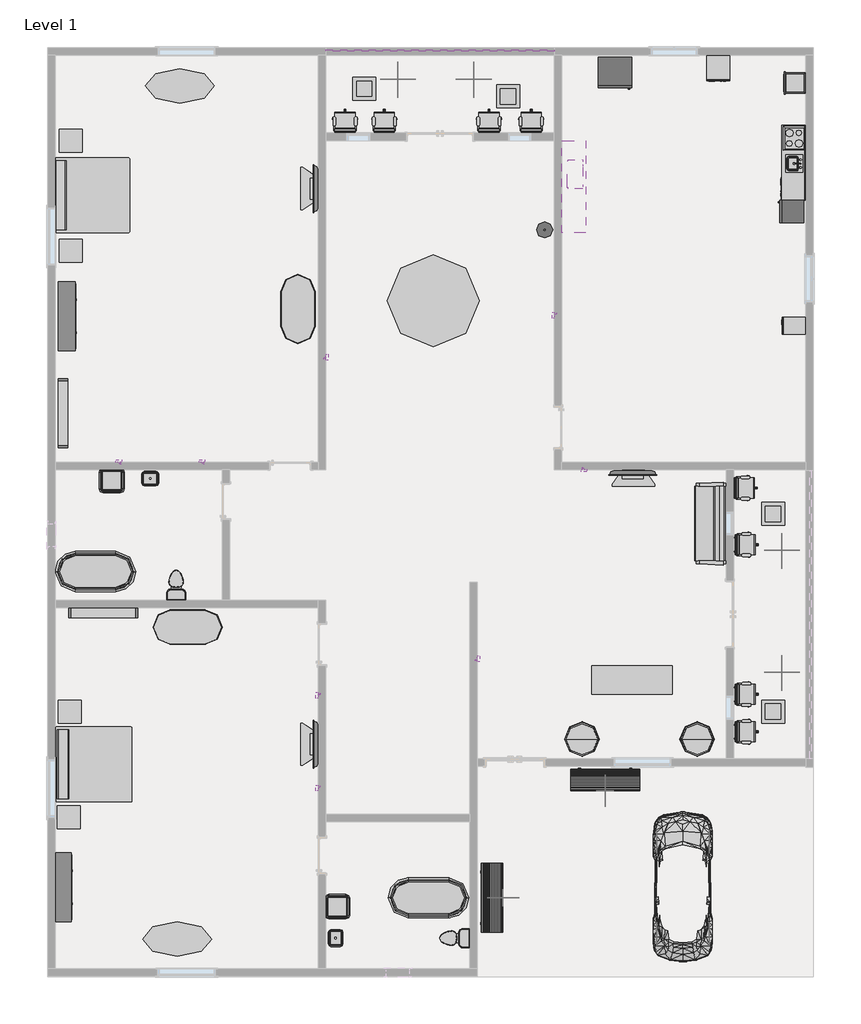
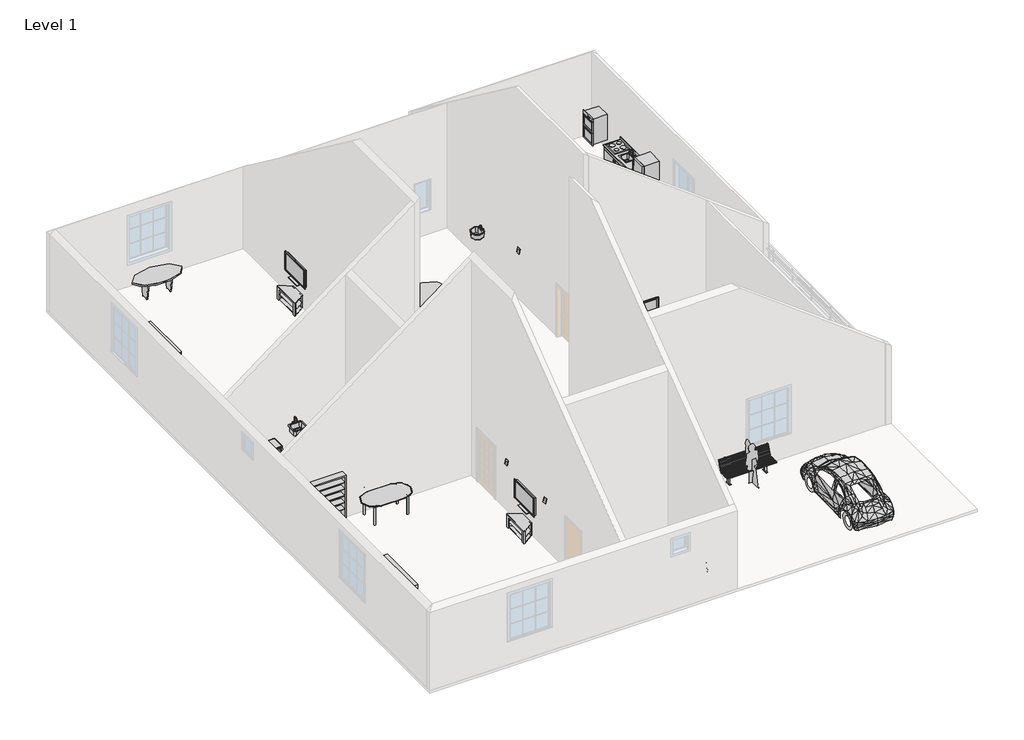
# One storey, part 2 of 2: 39 furniture elements, 20 proxies, 8 flow terminals, 8 geographic elements, 1 railing.
# Revit data of these elements (continued)
# Element 23 (IfcFlowTerminal, "Sink Vanity-Square : 20\" x 18\"") (continued)
#   Materials on its faces: "Porcelain, Linen", "Steel, Polished"
# Element 24 (IfcFlowTerminal, "Sink Vanity-Square : 20\" x 18\"")
#   Mark = "7"
#   Phase Created = New Construction
#   Materials on its faces: "Porcelain, Linen", "Steel, Polished"
# Element 25 (IfcFlowTerminal, "Toilet-Domestic-3D : Toilet-Domestic-3D")
#   Mark = "2"
#   Phase Created = New Construction
#   Materials on its faces: "Porcelain, Linen", "Laminate, Linen, Matte"
# Element 26 (IfcFlowTerminal, "Toilet-Domestic-3D : Toilet-Domestic-3D")
#   Mark = "5"
#   Phase Created = New Construction
#   Materials on its faces: "Porcelain, Linen", "Laminate, Linen, Matte"
# Element 27 (IfcFlowTerminal, "Tub-Free Standing-3D : 30\" x 60\"")
#   Mark = "1"
#   Phase Created = New Construction
#   Materials on its faces: "Porcelain, Ivory"
# Element 28 (IfcFlowTerminal, "Tub-Free Standing-3D : 30\" x 60\"")
#   Mark = "6"
#   Phase Created = New Construction
#   Materials on its faces: "Porcelain, Ivory"
# Elements 29, 30 (IfcFurniture, "Bed-Standard.0001 : King 78\" x 80\"")
#   Phase Created = New Construction
#   Materials on its faces: "Linen, White", "Steel, Chrome Plated"
# Elements 31, 32, 33, 34, 35, 36, 37, 38 (IfcFurniture, "Chair-Task Arms : Chair-Task Arms")
#   Phase Created = New Construction
#   Materials on its faces: "Plastic, Opaque Black", "Textile - Slate Blue"
# Element 39 (IfcFurniture, "Counter Top w Sink Hole : 24\" Depth")
#   Sink Opening Depth = 1' - 2"
#   Sink Location To Wall = 0' - 6"
#   Length = 6' - 6"
#   Sink Location = 3' - 4"
#   Sink Opening Width = 1' - 4"
#   Phase Created = New Construction
#   Materials on its faces: "Counter Top"
# Element 40 (IfcFurniture, "Counter Top w Sink Hole : Counter Top w Sink Hole")
#   Sink Opening Width = 2' - 3"
#   Sink Opening Depth = 1' - 3"
#   Sink Location To Wall = 0' - 6"
#   Sink Location = 2' - 0"
#   Length = 8' - 0"
#   Phase Created = New Construction
#   Materials on its faces: "Counter Top"
# Elements 41, 42 (IfcFurniture, "Dresser : 72\" x 60\" x 18\"")
#   Phase Created = New Construction
#   Materials on its faces: "Laminate, Ivory, Matte", "Cherry", "Laminate - Ivory, Glossy"
# Elements 43, 44 (IfcFurniture, "Shelving : 36\" x 10\" x 72\"")
#   Phase Created = New Construction
#   Materials on its faces: "Birch"
# Element 45 (IfcFurniture, "Sofa-Pensi : 84\"")
#   Phase Created = New Construction
#   Materials on its faces: "Cherry", "Linen, Beige", "Steel, Chrome Plated"
# Elements 46, 47, 48 (IfcFurniture, "TV - Flat Screen : 50\"")
#   Stand = yes
#   Phase Created = New Construction
#   Materials on its faces: "TV - Black", "TV - Glass", "TV - Screen"
# Elements 49, 50, 51 (IfcFurniture, "TV Stand : TV Stand")
#   Phase Created = New Construction
#   Materials on its faces: "Melamine - Gray", "Glass - Shelves"
# Elements 52, 53, 54, 55 (IfcFurniture, "Table-Coffee : 24\" x 24\" x 24\"")
#   Phase Created = New Construction
#   Materials on its faces: "Glass - Clear, Grey"
# Element 56 (IfcFurniture, "Table-Dining : 30\" x 84\" x 22\"")
#   Phase Created = New Construction
#   Materials on its faces: "Steel, Chrome Plated", "Glass - Clear, Grey"
# Elements 57, 58 (IfcFurniture, "Table-Dining Oval : 36\" x 72\"")
#   Phase Created = New Construction
#   Materials on its faces: "Steel, Chrome Plated", "Glass - Clear, Grey"
# Element 59 (IfcFurniture, "Table-Dining Round w Chairs : 84\" Diameter")
#   Phase Created = New Construction
#   Materials on its faces: "Pine", "Laminate, Linen, Matte"
# Elements 60, 61 (IfcFurniture, "Table-Ellipse : 72\" x 36\"")
#   Phase Created = New Construction
#   Materials on its faces: "Birch", "Laminate - Black"
# Elements 62, 63, 64, 65 (IfcFurniture, "Table-Night Stand : 24\" x 24\" x 30\"")
#   Phase Created = New Construction
#   Materials on its faces: "Birch", "Laminate, Ivory, Matte"
# Elements 66, 67 (IfcFurniture, "Table-Round : 36\" Diameter")
#   Phase Created = New Construction
#   Materials on its faces: "Steel, Chrome Plated", "Birch"
# Elements 68, 69 (IfcGeographicElement, "Park Bench : 72\"")
#   Phase Created = New Construction
#   Materials on its faces: "Wood - Teak", "Steel, Paint Finish, Dark Gray, Matte"
# Elements 70, 71, 72, 73 (IfcGeographicElement, "RPC Tree - Conifer : Chinese Juniper - 7'")
#   Phase Created = New Construction
# Elements 74, 75 (IfcGeographicElement, "Trash Can : Trash Can")
#   Phase Created = New Construction
#   Materials on its faces: "Plastic - Gray, Dark", "Plastic, Opaque Black"
# Element 76 (IfcRailing, "Guardrail - Pipe")
#   built-in parameter 1008621 = 4 (stored number, unit not read)
#   Phase Created = New Construction
# Materials
#   "Plastic, Opaque Black": class "Plastic", colour RGB 0 0 0, transparency 0.05, Description = "Plastic, generic, opaque black", Cost = 0
#   "Steel, Paint Finish, Ivory, Matte": class "Metal", colour RGB 247 247 239, transparency 0, Description = "Steel, paint finish, ivory, matte", Cost = 0
#   "Steel, Chrome Plated": class "Metal", colour RGB 17 17 17, transparency 0, Description = "Chromiuim plated steel", Cost = 0
#   "Steel, Polished": class "Metal", colour RGB 57 57 57, transparency 0, Description = "Polished steel", Cost = 0
#   "Steel, Paint Finish, Ivory, Glossy": class "Metal", colour RGB 247 247 239, transparency 0, Description = "Steel, paint finish, ivory, glossy", Cost = 0
#   "Cabinets": colour RGB 249 249 249, transparency 0
#   "Cabinets - Handles": class "Metal", colour RGB 57 57 57, transparency 0
#   "Laminate, Ivory, Matte": class "Plastic", colour RGB 247 247 239, transparency 0, Description = "Plastic Laminate - Ivory, Matte", Cost = 0
#   "Metal - Stainless Steel, Polished": class "Metal", colour RGB 216 216 216, transparency 0
#   "Porcelain, Linen": class "Ceramic", colour RGB 249 239 230, transparency 0, Description = "Porcelain, linen", Cost = 0
#   "Laminate, Linen, Matte": class "Plastic", colour RGB 249 239 230, transparency 0, Description = "Plastic Laminate - Linen, Matte", Cost = 0
#   "Porcelain, Ivory": class "Ceramic", colour RGB 247 247 239, transparency 0, Description = "Porcelain, ivory", Cost = 0
#   "Linen, White": class "Textile", colour RGB 247 247 239, transparency 0, Description = "Linen, white", Cost = 0
#   "Textile - Slate Blue": class "Fabric", colour RGB 98 102 118, transparency 0
#   "Laminate - Ivory, Glossy": colour RGB 247 247 239, transparency 0
#   "Cherry": class "Wood", colour RGB 226 177 128, transparency 0, Description = "Prunus Serotina", Cost = 0
#   "Birch": class "Wood", colour RGB 224 178 126, transparency 0, Description = "Betula Alleghaniensis", Cost = 0
#   "Linen, Beige": class "Textile", colour RGB 249 239 230, transparency 0, Description = "Linen, beige", Cost = 0
#   "Melamine - Gray": class "Wood", colour RGB 49 49 49, transparency 0
#   "Glass - Clear, Grey": class "Glass", colour RGB 252 255 255, transparency 0.64
#   "Pine": class "Wood", colour RGB 223 192 134, transparency 0, Description = "Pinus Echinata", Cost = 0
#   "Laminate - Black": colour RGB 0 0 0, transparency 0
#   "Wood - Teak": class "Wood", colour RGB 145 112 90, transparency 0
#   "Steel, Paint Finish, Dark Gray, Matte": class "Metal", colour RGB 98 98 98, transparency 0, Description = "Steel, paint finish, dark gray, matte", Cost = 0
#   "Glass": class "Glass", colour RGB 0 128 192, transparency 0.75, Description = "Soda Lime Glass", Cost = 0
#   "Steel": class "Metal", colour RGB 247 247 247, transparency 0, Description = "Steel, mill finish", Cost = 0
#   "Counter Top": class "Wood", colour RGB 226 177 128, transparency 0
#   "TV - Black": colour RGB 49 49 49, transparency 0
#   "TV - Glass": colour RGB 157 157 157, transparency 0.9
#   "TV - Screen": colour RGB 0 0 0, transparency 0
#   "Glass - Shelves": class "Glass", colour RGB 167 167 167, transparency 0.9
#   "Plastic - Gray, Dark": class "Plastic", colour RGB 134 134 134, transparency 0
